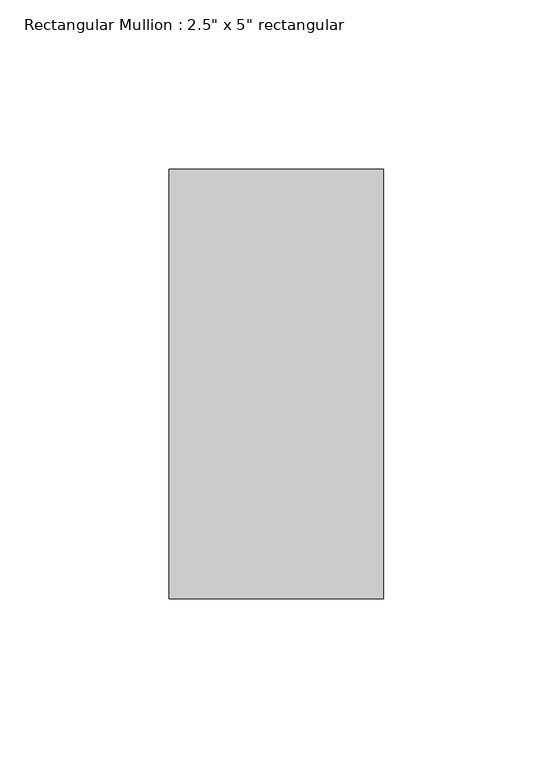
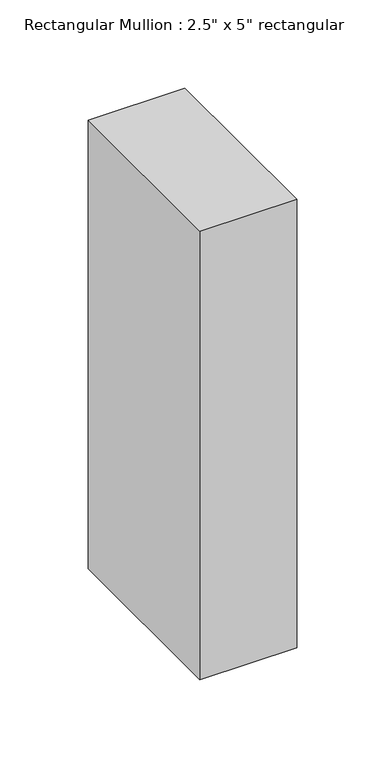
"""IFC4 building model written with IfcOpenShell, lengths in millimetres: member geometry."""

from ifc_helpers import new_model, si_unit, frame, origin, place, context, project, spatial, polyline, outline, extrude, source, transform, mapped, element, save


def member_5ad95953(model_context):
    return source(origin(), model_context, "Body", "SweptSolid", [
        extrude(outline(polyline([(0.0, 63.5), (0.0, -63.5), (-63.5, -63.5), (-63.5, 63.5), (0.0, 63.5)])), frame((0.0, 0.0, -311.15), z_axis=(0.0, 0.0, 1.0), x_axis=(1.0, 0.0, 0.0)), (0.0, 0.0, 1.0), 311.15),
    ])


if __name__ == "__main__":
    model = new_model("IFC4")
    model_context = context("Model", 3, world=origin())
    ifc_project = project(units=[si_unit("LENGTHUNIT", "METRE", prefix="MILLI")], contexts=[model_context])
    site = spatial("IfcSite", under=ifc_project)
    building = spatial("IfcBuilding", under=site)
    placement = place(None, origin())
    member_shape = member_5ad95953(model_context)
    element("IfcMember", 1, ObjectType="Rectangular Mullion : 2.5\" x 5\" rectangular", at=placement, inside=building, context=model_context, shape_type="MappedRepresentation", body=[
        mapped(member_shape, transform((0.0, 0.0, 0.0), x_axis=(1.0, 0.0, 0.0), y_axis=(0.0, 1.0, 0.0), z_axis=(0.0, 0.0, 1.0))),
    ])
    save(model, "model.ifc")

# Revit data of these elements
# Type "Rectangular Mullion : 2.5\" x 5\" rectangular"
#   built-in parameter 1007304 = 0.416667 (stored number, unit not read)
#   built-in parameter 1007301 = 0.104167 (stored number, unit not read)
#   built-in parameter 1007300 = 0.104167 (stored number, unit not read)
# Element 1 (IfcMember, "Rectangular Mullion : 2.5\" x 5\" rectangular")
#   Materials on its faces: "Door - Frame"
# Materials
#   "Door - Frame": colour RGB 118 70 51, transparency 0, Cost = 0
